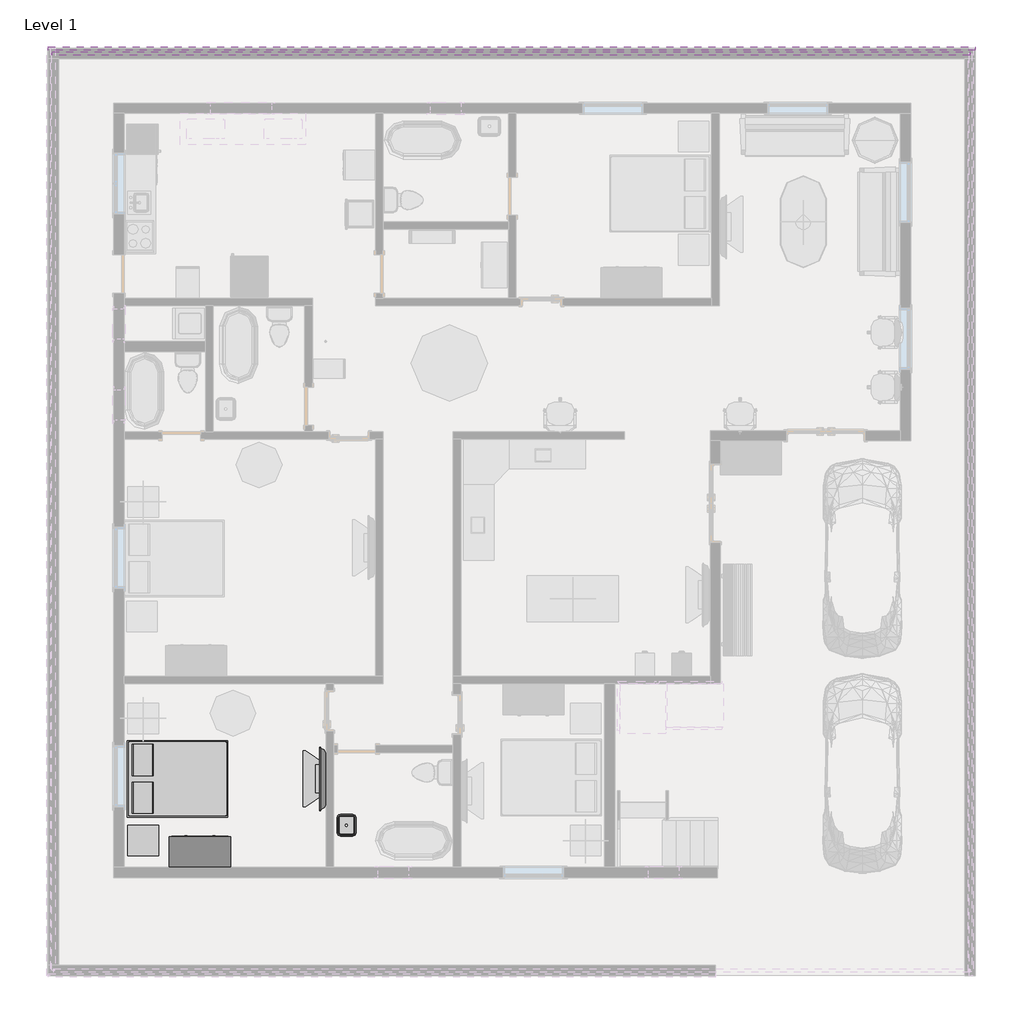
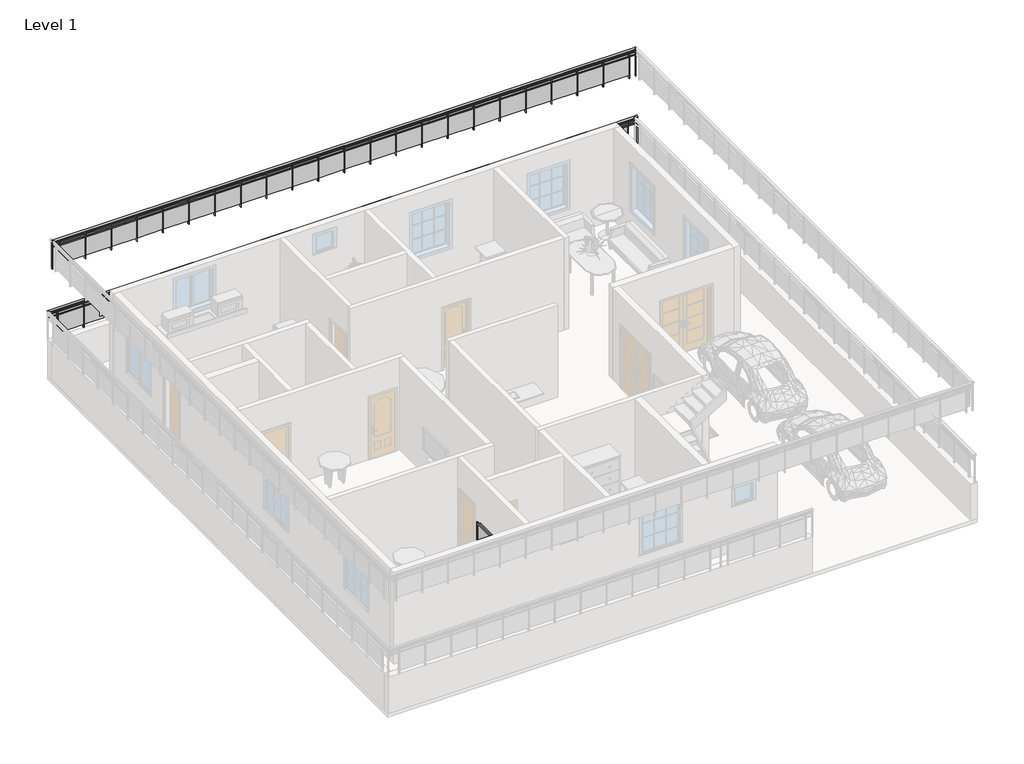
# One storey, part 5 of 6: 5 furniture elements, 2 railings, 1 flow terminal.
"""IFC4 building model written with IfcOpenShell, lengths in millimetres."""

from ifc_helpers import new_model, si_unit, point, frame, origin, place, context, project, spatial, polyline, ellipse_curve, trimmed, outline, extrude, transform, mapped, element, save
from ifc_brep_helpers import plane_surface, extruded_surface, advanced_brep
from components import flow_terminal_62a433f7, furniture_1d2926bd, furniture_9fa109b2, furniture_fdf74506, tv_stand_tv_stand_6ce107e5, furniture_5bc9ed15

model = new_model("IFC4")

# Units and contexts
model_context = context("Model", 3, world=origin())
ifc_project = project(units=[si_unit("LENGTHUNIT", "METRE", prefix="MILLI")], contexts=[model_context])

# Site, building, storey
site = spatial("IfcSite", under=ifc_project)
building = spatial("IfcBuilding", under=site)
storey = spatial("IfcBuildingStorey", under=building, Name="Level 1", Elevation=0.0)

# Flow terminal
placement = place(None, origin())
flow_terminal_shape = flow_terminal_62a433f7(model_context)
element("IfcFlowTerminal", 1, ObjectType="Sink Vanity-Square : 20\" x 18\"", at=placement, inside=storey, context=model_context, shape_type="MappedRepresentation", body=[
    mapped(flow_terminal_shape, transform((-1994.5948315, -1509.9134141, 609.6), x_axis=(0.0, 1.0000000000000004, 0.0), y_axis=(-1.0000000000000004, 0.0, 0.0), z_axis=(0.0, 0.0, 1.0))),
])

# Furniture
furniture_shape = furniture_1d2926bd(model_context)
element("IfcFurniture", 2, ObjectType="Bed-Box : Queen 60\" x 79\"", at=placement, inside=storey, context=model_context, shape_type="MappedRepresentation", body=[
    mapped(furniture_shape, transform((-5548.0082263, -906.2766325, 0.0), x_axis=(0.0, 1.0, 0.0), y_axis=(-1.0, 0.0, 0.0), z_axis=(0.0, 0.0, 1.0))),
])
furniture_2_shape = furniture_9fa109b2(model_context)
element("IfcFurniture", 3, ObjectType="Dresser : 48\" x 72\" x 24\"", at=placement, inside=storey, context=model_context, shape_type="MappedRepresentation", body=[
    mapped(furniture_2_shape, transform((-5136.3334924, -2390.7871276, 0.0), x_axis=(-1.0000000000000004, 0.0, 0.0), y_axis=(0.0, -1.0000000000000004, 0.0), z_axis=(0.0, 0.0, 1.0))),
])
furniture_3_shape = furniture_fdf74506(model_context)
element("IfcFurniture", 4, ObjectType="TV - Flat Screen : 50\"", at=placement, inside=storey, context=model_context, shape_type="MappedRepresentation", body=[
    mapped(furniture_3_shape, transform((-2411.0788562, -571.0686876, 914.4), x_axis=(0.0, -1.0, 0.0), y_axis=(1.0, 0.0, 0.0), z_axis=(0.0, 0.0, 1.0))),
])
tv_stand_tv_stand_shape = tv_stand_tv_stand_6ce107e5(model_context)
element("IfcFurniture", 5, ObjectType="TV Stand : TV Stand", at=placement, inside=storey, context=model_context, shape_type="MappedRepresentation", body=[
    mapped(tv_stand_tv_stand_shape, transform((-2352.5402326, -441.9361714, 0.0), x_axis=(0.0, -1.0, 0.0), y_axis=(1.0, 0.0, 0.0), z_axis=(0.0, 0.0, 1.0))),
])
furniture_4_shape = furniture_5bc9ed15(model_context)
element("IfcFurniture", 6, ObjectType="Table-Night Stand : 24\" x 24\" x 30\"", at=placement, inside=storey, context=model_context, shape_type="MappedRepresentation", body=[
    mapped(furniture_4_shape, transform((-6307.9123484, -2103.8241735, 0.0), x_axis=(1.0, 0.0, 0.0), y_axis=(0.0, 1.0, 0.0), z_axis=(0.0, 0.0, 1.0))),
])

# Railings
element("IfcRailing", 7, ObjectType="Glass Panel - Bottom Fill", at=placement, inside=storey, context=model_context, shape_type="SolidModel", body=[
    advanced_brep(
    [(10601.4597674, 13962.7633056, 2133.6), (10601.4597674, 14038.9633056, 2133.6), (-7889.7402326, 13962.7633056, 2133.6), (-7889.7402326, 14038.9633056, 2133.6)],
    [
        (0, 1, ellipse_curve(frame((10601.4597674, 14000.8633056, 2133.6), z_axis=(1.0, 0.0, 0.0), x_axis=(0.0, 1.0, 0.0)), 38.1, 28.575)),
        (1, 0, ellipse_curve(frame((10601.4597674, 14000.8633056, 2133.6), z_axis=(1.0, 0.0, 0.0), x_axis=(0.0, 1.0, 0.0)), 38.1, 28.575)),
        (2, 3, ellipse_curve(frame((-7889.7402326, 14000.8633056, 2133.6), z_axis=(-1.0, 0.0, 0.0), x_axis=(0.0, 1.0, 0.0)), 38.1, 28.575)),
        (3, 2, ellipse_curve(frame((-7889.7402326, 14000.8633056, 2133.6), z_axis=(-1.0, 0.0, 0.0), x_axis=(0.0, 1.0, 0.0)), 38.1, 28.575)),
        (0, 2),
        (3, 1),
    ],
    [
        plane_surface(frame((10601.4597674, 14000.8633056, 2133.6), z_axis=(1.0, 0.0, 0.0), x_axis=(0.0, -1.0, 0.0))),
        plane_surface(frame((-7889.7402326, 14000.8633056, 2133.6), z_axis=(-1.0, 0.0, 0.0), x_axis=(0.0, -1.0, 0.0))),
        extruded_surface(trimmed(ellipse_curve(frame((-7889.7402326, 14000.8633056, 2133.6), z_axis=(1.0, 0.0, 0.0), x_axis=(0.0, 1.0, 0.0)), 38.1, 28.575), [point((-7889.7402326, 13962.7633056, 2133.6))], [point((-7889.7402326, 14038.9633056, 2133.6))], True, "CARTESIAN"), (18491.2, 0.0, 0.0), 18491.2),
        extruded_surface(trimmed(ellipse_curve(frame((-7889.7402326, 14000.8633056, 2133.6), z_axis=(1.0, 0.0, 0.0), x_axis=(0.0, 1.0, 0.0)), 38.1, 28.575), [point((-7889.7402326, 14038.9633056, 2133.6))], [point((-7889.7402326, 13962.7633056, 2133.6))], True, "CARTESIAN"), (18491.2, 0.0, 0.0), 18491.2),
    ],
    [
        (0, [[1, 2]]),
        (1, [[3, 4]]),
        (2, [[-1, 5, -4, 6]]),
        (3, [[-2, -6, -3, -5]]),
    ],
),
    extrude(outline(polyline([(10601.4597674, 14013.5633056), (10601.4597674, 13988.1633056), (-7889.7402326, 13988.1633056), (-7889.7402326, 14013.5633056), (10601.4597674, 14013.5633056)])), frame((0.0, 0.0, 2019.3), z_axis=(0.0, 0.0, 1.0), x_axis=(1.0, 0.0, 0.0)), (0.0, 0.0, 1.0), 25.4),
    extrude(outline(polyline([(10601.4597674, 14013.5633056), (10601.4597674, 13988.1633056), (-7889.7402326, 13988.1633056), (-7889.7402326, 14013.5633056), (10601.4597674, 14013.5633056)])), frame((0.0, 0.0, 1917.7), z_axis=(0.0, 0.0, 1.0), x_axis=(1.0, 0.0, 0.0)), (0.0, 0.0, 1.0), 25.4),
    extrude(outline(polyline([(-7578.5902326, 14026.2633056), (-7578.5902326, 13975.4633056), (-7591.2902326, 13975.4633056), (-7591.2902326, 14026.2633056), (-7578.5902326, 14026.2633056)])), frame((0.0, 0.0, 1219.2), z_axis=(0.0, 0.0, 1.0), x_axis=(1.0, 0.0, 0.0)), (0.0, 0.0, 1.0), 885.6788223),
    extrude(outline(polyline([(-6772.1402326, 13994.3281486), (-7584.9402326, 13994.3281486), (-7584.9402326, 14000.6781486), (-6772.1402326, 14000.6781486), (-6772.1402326, 13994.3281486)])), frame((0.0, 0.0, 1320.8), z_axis=(0.0, 0.0, 1.0), x_axis=(1.0, 0.0, 0.0)), (0.0, 0.0, 1.0), 596.9),
    extrude(outline(polyline([(-6765.7902326, 14026.2633056), (-6765.7902326, 13975.4633056), (-6778.4902326, 13975.4633056), (-6778.4902326, 14026.2633056), (-6765.7902326, 14026.2633056)])), frame((0.0, 0.0, 1219.2), z_axis=(0.0, 0.0, 1.0), x_axis=(1.0, 0.0, 0.0)), (0.0, 0.0, 1.0), 885.6788223),
    extrude(outline(polyline([(-5959.3402326, 13994.3281486), (-6772.1402326, 13994.3281486), (-6772.1402326, 14000.6781486), (-5959.3402326, 14000.6781486), (-5959.3402326, 13994.3281486)])), frame((0.0, 0.0, 1320.8), z_axis=(0.0, 0.0, 1.0), x_axis=(1.0, 0.0, 0.0)), (0.0, 0.0, 1.0), 596.9),
    extrude(outline(polyline([(-5952.9902326, 14026.2633056), (-5952.9902326, 13975.4633056), (-5965.6902326, 13975.4633056), (-5965.6902326, 14026.2633056), (-5952.9902326, 14026.2633056)])), frame((0.0, 0.0, 1219.2), z_axis=(0.0, 0.0, 1.0), x_axis=(1.0, 0.0, 0.0)), (0.0, 0.0, 1.0), 885.6788223),
    extrude(outline(polyline([(-5146.5402326, 13994.3281486), (-5959.3402326, 13994.3281486), (-5959.3402326, 14000.6781486), (-5146.5402326, 14000.6781486), (-5146.5402326, 13994.3281486)])), frame((0.0, 0.0, 1320.8), z_axis=(0.0, 0.0, 1.0), x_axis=(1.0, 0.0, 0.0)), (0.0, 0.0, 1.0), 596.9),
    extrude(outline(polyline([(-5140.1902326, 14026.2633056), (-5140.1902326, 13975.4633056), (-5152.8902326, 13975.4633056), (-5152.8902326, 14026.2633056), (-5140.1902326, 14026.2633056)])), frame((0.0, 0.0, 1219.2), z_axis=(0.0, 0.0, 1.0), x_axis=(1.0, 0.0, 0.0)), (0.0, 0.0, 1.0), 885.6788223),
    extrude(outline(polyline([(-4333.7402326, 13994.3281486), (-5146.5402326, 13994.3281486), (-5146.5402326, 14000.6781486), (-4333.7402326, 14000.6781486), (-4333.7402326, 13994.3281486)])), frame((0.0, 0.0, 1320.8), z_axis=(0.0, 0.0, 1.0), x_axis=(1.0, 0.0, 0.0)), (0.0, 0.0, 1.0), 596.9),
    extrude(outline(polyline([(-4327.3902326, 14026.2633056), (-4327.3902326, 13975.4633056), (-4340.0902326, 13975.4633056), (-4340.0902326, 14026.2633056), (-4327.3902326, 14026.2633056)])), frame((0.0, 0.0, 1219.2), z_axis=(0.0, 0.0, 1.0), x_axis=(1.0, 0.0, 0.0)), (0.0, 0.0, 1.0), 885.6788223),
    extrude(outline(polyline([(-3520.9402326, 13994.3281486), (-4333.7402326, 13994.3281486), (-4333.7402326, 14000.6781486), (-3520.9402326, 14000.6781486), (-3520.9402326, 13994.3281486)])), frame((0.0, 0.0, 1320.8), z_axis=(0.0, 0.0, 1.0), x_axis=(1.0, 0.0, 0.0)), (0.0, 0.0, 1.0), 596.9),
    extrude(outline(polyline([(-3514.5902326, 14026.2633056), (-3514.5902326, 13975.4633056), (-3527.2902326, 13975.4633056), (-3527.2902326, 14026.2633056), (-3514.5902326, 14026.2633056)])), frame((0.0, 0.0, 1219.2), z_axis=(0.0, 0.0, 1.0), x_axis=(1.0, 0.0, 0.0)), (0.0, 0.0, 1.0), 885.6788223),
    extrude(outline(polyline([(-2708.1402326, 13994.3281486), (-3520.9402326, 13994.3281486), (-3520.9402326, 14000.6781486), (-2708.1402326, 14000.6781486), (-2708.1402326, 13994.3281486)])), frame((0.0, 0.0, 1320.8), z_axis=(0.0, 0.0, 1.0), x_axis=(1.0, 0.0, 0.0)), (0.0, 0.0, 1.0), 596.9),
    extrude(outline(polyline([(-2701.7902326, 14026.2633056), (-2701.7902326, 13975.4633056), (-2714.4902326, 13975.4633056), (-2714.4902326, 14026.2633056), (-2701.7902326, 14026.2633056)])), frame((0.0, 0.0, 1219.2), z_axis=(0.0, 0.0, 1.0), x_axis=(1.0, 0.0, 0.0)), (0.0, 0.0, 1.0), 885.6788223),
    extrude(outline(polyline([(-1895.3402326, 13994.3281486), (-2708.1402326, 13994.3281486), (-2708.1402326, 14000.6781486), (-1895.3402326, 14000.6781486), (-1895.3402326, 13994.3281486)])), frame((0.0, 0.0, 1320.8), z_axis=(0.0, 0.0, 1.0), x_axis=(1.0, 0.0, 0.0)), (0.0, 0.0, 1.0), 596.9),
    extrude(outline(polyline([(-1888.9902326, 14026.2633056), (-1888.9902326, 13975.4633056), (-1901.6902326, 13975.4633056), (-1901.6902326, 14026.2633056), (-1888.9902326, 14026.2633056)])), frame((0.0, 0.0, 1219.2), z_axis=(0.0, 0.0, 1.0), x_axis=(1.0, 0.0, 0.0)), (0.0, 0.0, 1.0), 885.6788223),
    extrude(outline(polyline([(-1082.5402326, 13994.3281486), (-1895.3402326, 13994.3281486), (-1895.3402326, 14000.6781486), (-1082.5402326, 14000.6781486), (-1082.5402326, 13994.3281486)])), frame((0.0, 0.0, 1320.8), z_axis=(0.0, 0.0, 1.0), x_axis=(1.0, 0.0, 0.0)), (0.0, 0.0, 1.0), 596.9),
    extrude(outline(polyline([(-1076.1902326, 14026.2633056), (-1076.1902326, 13975.4633056), (-1088.8902326, 13975.4633056), (-1088.8902326, 14026.2633056), (-1076.1902326, 14026.2633056)])), frame((0.0, 0.0, 1219.2), z_axis=(0.0, 0.0, 1.0), x_axis=(1.0, 0.0, 0.0)), (0.0, 0.0, 1.0), 885.6788223),
    extrude(outline(polyline([(-269.7402326, 13994.3281486), (-1082.5402326, 13994.3281486), (-1082.5402326, 14000.6781486), (-269.7402326, 14000.6781486), (-269.7402326, 13994.3281486)])), frame((0.0, 0.0, 1320.8), z_axis=(0.0, 0.0, 1.0), x_axis=(1.0, 0.0, 0.0)), (0.0, 0.0, 1.0), 596.9),
    extrude(outline(polyline([(-263.3902326, 14026.2633056), (-263.3902326, 13975.4633056), (-276.0902326, 13975.4633056), (-276.0902326, 14026.2633056), (-263.3902326, 14026.2633056)])), frame((0.0, 0.0, 1219.2), z_axis=(0.0, 0.0, 1.0), x_axis=(1.0, 0.0, 0.0)), (0.0, 0.0, 1.0), 885.6788223),
    extrude(outline(polyline([(543.0597674, 13994.3281486), (-269.7402326, 13994.3281486), (-269.7402326, 14000.6781486), (543.0597674, 14000.6781486), (543.0597674, 13994.3281486)])), frame((0.0, 0.0, 1320.8), z_axis=(0.0, 0.0, 1.0), x_axis=(1.0, 0.0, 0.0)), (0.0, 0.0, 1.0), 596.9),
    extrude(outline(polyline([(549.4097674, 14026.2633056), (549.4097674, 13975.4633056), (536.7097674, 13975.4633056), (536.7097674, 14026.2633056), (549.4097674, 14026.2633056)])), frame((0.0, 0.0, 1219.2), z_axis=(0.0, 0.0, 1.0), x_axis=(1.0, 0.0, 0.0)), (0.0, 0.0, 1.0), 885.6788223),
    extrude(outline(polyline([(1355.8597674, 13994.3281486), (543.0597674, 13994.3281486), (543.0597674, 14000.6781486), (1355.8597674, 14000.6781486), (1355.8597674, 13994.3281486)])), frame((0.0, 0.0, 1320.8), z_axis=(0.0, 0.0, 1.0), x_axis=(1.0, 0.0, 0.0)), (0.0, 0.0, 1.0), 596.9),
    extrude(outline(polyline([(1362.2097674, 14026.2633056), (1362.2097674, 13975.4633056), (1349.5097674, 13975.4633056), (1349.5097674, 14026.2633056), (1362.2097674, 14026.2633056)])), frame((0.0, 0.0, 1219.2), z_axis=(0.0, 0.0, 1.0), x_axis=(1.0, 0.0, 0.0)), (0.0, 0.0, 1.0), 885.6788223),
    extrude(outline(polyline([(2168.6597674, 13994.3281486), (1355.8597674, 13994.3281486), (1355.8597674, 14000.6781486), (2168.6597674, 14000.6781486), (2168.6597674, 13994.3281486)])), frame((0.0, 0.0, 1320.8), z_axis=(0.0, 0.0, 1.0), x_axis=(1.0, 0.0, 0.0)), (0.0, 0.0, 1.0), 596.9),
    extrude(outline(polyline([(2175.0097674, 14026.2633056), (2175.0097674, 13975.4633056), (2162.3097674, 13975.4633056), (2162.3097674, 14026.2633056), (2175.0097674, 14026.2633056)])), frame((0.0, 0.0, 1219.2), z_axis=(0.0, 0.0, 1.0), x_axis=(1.0, 0.0, 0.0)), (0.0, 0.0, 1.0), 885.6788223),
    extrude(outline(polyline([(2981.4597674, 13994.3281486), (2168.6597674, 13994.3281486), (2168.6597674, 14000.6781486), (2981.4597674, 14000.6781486), (2981.4597674, 13994.3281486)])), frame((0.0, 0.0, 1320.8), z_axis=(0.0, 0.0, 1.0), x_axis=(1.0, 0.0, 0.0)), (0.0, 0.0, 1.0), 596.9),
    extrude(outline(polyline([(2987.8097674, 14026.2633056), (2987.8097674, 13975.4633056), (2975.1097674, 13975.4633056), (2975.1097674, 14026.2633056), (2987.8097674, 14026.2633056)])), frame((0.0, 0.0, 1219.2), z_axis=(0.0, 0.0, 1.0), x_axis=(1.0, 0.0, 0.0)), (0.0, 0.0, 1.0), 885.6788223),
    extrude(outline(polyline([(3794.2597674, 13994.3281486), (2981.4597674, 13994.3281486), (2981.4597674, 14000.6781486), (3794.2597674, 14000.6781486), (3794.2597674, 13994.3281486)])), frame((0.0, 0.0, 1320.8), z_axis=(0.0, 0.0, 1.0), x_axis=(1.0, 0.0, 0.0)), (0.0, 0.0, 1.0), 596.9),
    extrude(outline(polyline([(3800.6097674, 14026.2633056), (3800.6097674, 13975.4633056), (3787.9097674, 13975.4633056), (3787.9097674, 14026.2633056), (3800.6097674, 14026.2633056)])), frame((0.0, 0.0, 1219.2), z_axis=(0.0, 0.0, 1.0), x_axis=(1.0, 0.0, 0.0)), (0.0, 0.0, 1.0), 885.6788223),
    extrude(outline(polyline([(4607.0597674, 13994.3281486), (3794.2597674, 13994.3281486), (3794.2597674, 14000.6781486), (4607.0597674, 14000.6781486), (4607.0597674, 13994.3281486)])), frame((0.0, 0.0, 1320.8), z_axis=(0.0, 0.0, 1.0), x_axis=(1.0, 0.0, 0.0)), (0.0, 0.0, 1.0), 596.9),
    extrude(outline(polyline([(4613.4097674, 14026.2633056), (4613.4097674, 13975.4633056), (4600.7097674, 13975.4633056), (4600.7097674, 14026.2633056), (4613.4097674, 14026.2633056)])), frame((0.0, 0.0, 1219.2), z_axis=(0.0, 0.0, 1.0), x_axis=(1.0, 0.0, 0.0)), (0.0, 0.0, 1.0), 885.6788223),
    extrude(outline(polyline([(5419.8597674, 13994.3281486), (4607.0597674, 13994.3281486), (4607.0597674, 14000.6781486), (5419.8597674, 14000.6781486), (5419.8597674, 13994.3281486)])), frame((0.0, 0.0, 1320.8), z_axis=(0.0, 0.0, 1.0), x_axis=(1.0, 0.0, 0.0)), (0.0, 0.0, 1.0), 596.9),
    extrude(outline(polyline([(5426.2097674, 14026.2633056), (5426.2097674, 13975.4633056), (5413.5097674, 13975.4633056), (5413.5097674, 14026.2633056), (5426.2097674, 14026.2633056)])), frame((0.0, 0.0, 1219.2), z_axis=(0.0, 0.0, 1.0), x_axis=(1.0, 0.0, 0.0)), (0.0, 0.0, 1.0), 885.6788223),
    extrude(outline(polyline([(6232.6597674, 13994.3281486), (5419.8597674, 13994.3281486), (5419.8597674, 14000.6781486), (6232.6597674, 14000.6781486), (6232.6597674, 13994.3281486)])), frame((0.0, 0.0, 1320.8), z_axis=(0.0, 0.0, 1.0), x_axis=(1.0, 0.0, 0.0)), (0.0, 0.0, 1.0), 596.9),
    extrude(outline(polyline([(6239.0097674, 14026.2633056), (6239.0097674, 13975.4633056), (6226.3097674, 13975.4633056), (6226.3097674, 14026.2633056), (6239.0097674, 14026.2633056)])), frame((0.0, 0.0, 1219.2), z_axis=(0.0, 0.0, 1.0), x_axis=(1.0, 0.0, 0.0)), (0.0, 0.0, 1.0), 885.6788223),
    extrude(outline(polyline([(7045.4597674, 13994.3281486), (6232.6597674, 13994.3281486), (6232.6597674, 14000.6781486), (7045.4597674, 14000.6781486), (7045.4597674, 13994.3281486)])), frame((0.0, 0.0, 1320.8), z_axis=(0.0, 0.0, 1.0), x_axis=(1.0, 0.0, 0.0)), (0.0, 0.0, 1.0), 596.9),
    extrude(outline(polyline([(7051.8097674, 14026.2633056), (7051.8097674, 13975.4633056), (7039.1097674, 13975.4633056), (7039.1097674, 14026.2633056), (7051.8097674, 14026.2633056)])), frame((0.0, 0.0, 1219.2), z_axis=(0.0, 0.0, 1.0), x_axis=(1.0, 0.0, 0.0)), (0.0, 0.0, 1.0), 885.6788223),
    extrude(outline(polyline([(7858.2597674, 13994.3281486), (7045.4597674, 13994.3281486), (7045.4597674, 14000.6781486), (7858.2597674, 14000.6781486), (7858.2597674, 13994.3281486)])), frame((0.0, 0.0, 1320.8), z_axis=(0.0, 0.0, 1.0), x_axis=(1.0, 0.0, 0.0)), (0.0, 0.0, 1.0), 596.9),
    extrude(outline(polyline([(7864.6097674, 14026.2633056), (7864.6097674, 13975.4633056), (7851.9097674, 13975.4633056), (7851.9097674, 14026.2633056), (7864.6097674, 14026.2633056)])), frame((0.0, 0.0, 1219.2), z_axis=(0.0, 0.0, 1.0), x_axis=(1.0, 0.0, 0.0)), (0.0, 0.0, 1.0), 885.6788223),
    extrude(outline(polyline([(8671.0597674, 13994.3281486), (7858.2597674, 13994.3281486), (7858.2597674, 14000.6781486), (8671.0597674, 14000.6781486), (8671.0597674, 13994.3281486)])), frame((0.0, 0.0, 1320.8), z_axis=(0.0, 0.0, 1.0), x_axis=(1.0, 0.0, 0.0)), (0.0, 0.0, 1.0), 596.9),
    extrude(outline(polyline([(8677.4097674, 14026.2633056), (8677.4097674, 13975.4633056), (8664.7097674, 13975.4633056), (8664.7097674, 14026.2633056), (8677.4097674, 14026.2633056)])), frame((0.0, 0.0, 1219.2), z_axis=(0.0, 0.0, 1.0), x_axis=(1.0, 0.0, 0.0)), (0.0, 0.0, 1.0), 885.6788223),
    extrude(outline(polyline([(9483.8597674, 13994.3281486), (8671.0597674, 13994.3281486), (8671.0597674, 14000.6781486), (9483.8597674, 14000.6781486), (9483.8597674, 13994.3281486)])), frame((0.0, 0.0, 1320.8), z_axis=(0.0, 0.0, 1.0), x_axis=(1.0, 0.0, 0.0)), (0.0, 0.0, 1.0), 596.9),
    extrude(outline(polyline([(9490.2097674, 14026.2633056), (9490.2097674, 13975.4633056), (9477.5097674, 13975.4633056), (9477.5097674, 14026.2633056), (9490.2097674, 14026.2633056)])), frame((0.0, 0.0, 1219.2), z_axis=(0.0, 0.0, 1.0), x_axis=(1.0, 0.0, 0.0)), (0.0, 0.0, 1.0), 885.6788223),
    extrude(outline(polyline([(10296.6597674, 13994.3281486), (9483.8597674, 13994.3281486), (9483.8597674, 14000.6781486), (10296.6597674, 14000.6781486), (10296.6597674, 13994.3281486)])), frame((0.0, 0.0, 1320.8), z_axis=(0.0, 0.0, 1.0), x_axis=(1.0, 0.0, 0.0)), (0.0, 0.0, 1.0), 596.9),
    extrude(outline(polyline([(10303.0097674, 14026.2633056), (10303.0097674, 13975.4633056), (10290.3097674, 13975.4633056), (10290.3097674, 14026.2633056), (10303.0097674, 14026.2633056)])), frame((0.0, 0.0, 1219.2), z_axis=(0.0, 0.0, 1.0), x_axis=(1.0, 0.0, 0.0)), (0.0, 0.0, 1.0), 885.6788223),
    extrude(outline(polyline([(-7877.0402326, 14010.3883056), (-7877.0402326, 13991.3383056), (-7896.0902326, 13991.3383056), (-7896.0902326, 14010.3883056), (-7877.0402326, 14010.3883056)])), frame((0.0, 0.0, 1219.2), z_axis=(0.0, 0.0, 1.0), x_axis=(1.0, 0.0, 0.0)), (0.0, 0.0, 1.0), 885.6788223),
    extrude(outline(polyline([(10607.8097674, 14010.3883056), (10607.8097674, 13991.3383056), (10588.7597674, 13991.3383056), (10588.7597674, 14010.3883056), (10607.8097674, 14010.3883056)])), frame((0.0, 0.0, 1219.2), z_axis=(0.0, 0.0, 1.0), x_axis=(1.0, 0.0, 0.0)), (0.0, 0.0, 1.0), 885.6788223),
])
element("IfcRailing", 8, ObjectType="Glass Panel - Bottom Fill", at=placement, inside=storey, context=model_context, shape_type="SolidModel", body=[
    advanced_brep(
    [(10499.8597674, 13861.1633056, 4495.8), (10499.8597674, 13937.3633056, 4495.8), (-7813.5402326, 13861.1633056, 4495.8), (-7813.5402326, 13937.3633056, 4495.8)],
    [
        (0, 1, ellipse_curve(frame((10499.8597674, 13899.2633056, 4495.8), z_axis=(1.0, 0.0, 0.0), x_axis=(0.0, 1.0, 0.0)), 38.1, 28.575)),
        (1, 0, ellipse_curve(frame((10499.8597674, 13899.2633056, 4495.8), z_axis=(1.0, 0.0, 0.0), x_axis=(0.0, 1.0, 0.0)), 38.1, 28.575)),
        (2, 3, ellipse_curve(frame((-7813.5402326, 13899.2633056, 4495.8), z_axis=(-1.0, 0.0, 0.0), x_axis=(0.0, 1.0, 0.0)), 38.1, 28.575)),
        (3, 2, ellipse_curve(frame((-7813.5402326, 13899.2633056, 4495.8), z_axis=(-1.0, 0.0, 0.0), x_axis=(0.0, 1.0, 0.0)), 38.1, 28.575)),
        (0, 2),
        (3, 1),
    ],
    [
        plane_surface(frame((10499.8597674, 13899.2633056, 4495.8), z_axis=(1.0, 0.0, 0.0), x_axis=(0.0, -1.0, 0.0))),
        plane_surface(frame((-7813.5402326, 13899.2633056, 4495.8), z_axis=(-1.0, 0.0, 0.0), x_axis=(0.0, -1.0, 0.0))),
        extruded_surface(trimmed(ellipse_curve(frame((-7813.5402326, 13899.2633056, 4495.8), z_axis=(1.0, 0.0, 0.0), x_axis=(0.0, 1.0, 0.0)), 38.1, 28.575), [point((-7813.5402326, 13861.1633056, 4495.8))], [point((-7813.5402326, 13937.3633056, 4495.8))], True, "CARTESIAN"), (18313.4, 0.0, 0.0), 18313.4),
        extruded_surface(trimmed(ellipse_curve(frame((-7813.5402326, 13899.2633056, 4495.8), z_axis=(1.0, 0.0, 0.0), x_axis=(0.0, 1.0, 0.0)), 38.1, 28.575), [point((-7813.5402326, 13937.3633056, 4495.8))], [point((-7813.5402326, 13861.1633056, 4495.8))], True, "CARTESIAN"), (18313.4, 0.0, 0.0), 18313.4),
    ],
    [
        (0, [[1, 2]]),
        (1, [[3, 4]]),
        (2, [[-1, 5, -4, 6]]),
        (3, [[-2, -6, -3, -5]]),
    ],
),
    extrude(outline(polyline([(10499.8597674, 13911.9633056), (10499.8597674, 13886.5633056), (-7813.5402326, 13886.5633056), (-7813.5402326, 13911.9633056), (10499.8597674, 13911.9633056)])), frame((0.0, 0.0, 4381.5), z_axis=(0.0, 0.0, 1.0), x_axis=(1.0, 0.0, 0.0)), (0.0, 0.0, 1.0), 25.4),
    extrude(outline(polyline([(10499.8597674, 13911.9633056), (10499.8597674, 13886.5633056), (-7813.5402326, 13886.5633056), (-7813.5402326, 13911.9633056), (10499.8597674, 13911.9633056)])), frame((0.0, 0.0, 4279.9), z_axis=(0.0, 0.0, 1.0), x_axis=(1.0, 0.0, 0.0)), (0.0, 0.0, 1.0), 25.4),
    extrude(outline(polyline([(-7591.2902326, 13924.6633056), (-7591.2902326, 13873.8633056), (-7603.9902326, 13873.8633056), (-7603.9902326, 13924.6633056), (-7591.2902326, 13924.6633056)])), frame((0.0, 0.0, 3581.4), z_axis=(0.0, 0.0, 1.0), x_axis=(1.0, 0.0, 0.0)), (0.0, 0.0, 1.0), 885.6788223),
    extrude(outline(polyline([(-6784.8402326, 13892.7281486), (-7597.6402326, 13892.7281486), (-7597.6402326, 13899.0781486), (-6784.8402326, 13899.0781486), (-6784.8402326, 13892.7281486)])), frame((0.0, 0.0, 3683.0), z_axis=(0.0, 0.0, 1.0), x_axis=(1.0, 0.0, 0.0)), (0.0, 0.0, 1.0), 596.9),
    extrude(outline(polyline([(-6778.4902326, 13924.6633056), (-6778.4902326, 13873.8633056), (-6791.1902326, 13873.8633056), (-6791.1902326, 13924.6633056), (-6778.4902326, 13924.6633056)])), frame((0.0, 0.0, 3581.4), z_axis=(0.0, 0.0, 1.0), x_axis=(1.0, 0.0, 0.0)), (0.0, 0.0, 1.0), 885.6788223),
    extrude(outline(polyline([(-5972.0402326, 13892.7281486), (-6784.8402326, 13892.7281486), (-6784.8402326, 13899.0781486), (-5972.0402326, 13899.0781486), (-5972.0402326, 13892.7281486)])), frame((0.0, 0.0, 3683.0), z_axis=(0.0, 0.0, 1.0), x_axis=(1.0, 0.0, 0.0)), (0.0, 0.0, 1.0), 596.9),
    extrude(outline(polyline([(-5965.6902326, 13924.6633056), (-5965.6902326, 13873.8633056), (-5978.3902326, 13873.8633056), (-5978.3902326, 13924.6633056), (-5965.6902326, 13924.6633056)])), frame((0.0, 0.0, 3581.4), z_axis=(0.0, 0.0, 1.0), x_axis=(1.0, 0.0, 0.0)), (0.0, 0.0, 1.0), 885.6788223),
    extrude(outline(polyline([(-5159.2402326, 13892.7281486), (-5972.0402326, 13892.7281486), (-5972.0402326, 13899.0781486), (-5159.2402326, 13899.0781486), (-5159.2402326, 13892.7281486)])), frame((0.0, 0.0, 3683.0), z_axis=(0.0, 0.0, 1.0), x_axis=(1.0, 0.0, 0.0)), (0.0, 0.0, 1.0), 596.9),
    extrude(outline(polyline([(-5152.8902326, 13924.6633056), (-5152.8902326, 13873.8633056), (-5165.5902326, 13873.8633056), (-5165.5902326, 13924.6633056), (-5152.8902326, 13924.6633056)])), frame((0.0, 0.0, 3581.4), z_axis=(0.0, 0.0, 1.0), x_axis=(1.0, 0.0, 0.0)), (0.0, 0.0, 1.0), 885.6788223),
    extrude(outline(polyline([(-4346.4402326, 13892.7281486), (-5159.2402326, 13892.7281486), (-5159.2402326, 13899.0781486), (-4346.4402326, 13899.0781486), (-4346.4402326, 13892.7281486)])), frame((0.0, 0.0, 3683.0), z_axis=(0.0, 0.0, 1.0), x_axis=(1.0, 0.0, 0.0)), (0.0, 0.0, 1.0), 596.9),
    extrude(outline(polyline([(-4340.0902326, 13924.6633056), (-4340.0902326, 13873.8633056), (-4352.7902326, 13873.8633056), (-4352.7902326, 13924.6633056), (-4340.0902326, 13924.6633056)])), frame((0.0, 0.0, 3581.4), z_axis=(0.0, 0.0, 1.0), x_axis=(1.0, 0.0, 0.0)), (0.0, 0.0, 1.0), 885.6788223),
    extrude(outline(polyline([(-3533.6402326, 13892.7281486), (-4346.4402326, 13892.7281486), (-4346.4402326, 13899.0781486), (-3533.6402326, 13899.0781486), (-3533.6402326, 13892.7281486)])), frame((0.0, 0.0, 3683.0), z_axis=(0.0, 0.0, 1.0), x_axis=(1.0, 0.0, 0.0)), (0.0, 0.0, 1.0), 596.9),
    extrude(outline(polyline([(-3527.2902326, 13924.6633056), (-3527.2902326, 13873.8633056), (-3539.9902326, 13873.8633056), (-3539.9902326, 13924.6633056), (-3527.2902326, 13924.6633056)])), frame((0.0, 0.0, 3581.4), z_axis=(0.0, 0.0, 1.0), x_axis=(1.0, 0.0, 0.0)), (0.0, 0.0, 1.0), 885.6788223),
    extrude(outline(polyline([(-2720.8402326, 13892.7281486), (-3533.6402326, 13892.7281486), (-3533.6402326, 13899.0781486), (-2720.8402326, 13899.0781486), (-2720.8402326, 13892.7281486)])), frame((0.0, 0.0, 3683.0), z_axis=(0.0, 0.0, 1.0), x_axis=(1.0, 0.0, 0.0)), (0.0, 0.0, 1.0), 596.9),
    extrude(outline(polyline([(-2714.4902326, 13924.6633056), (-2714.4902326, 13873.8633056), (-2727.1902326, 13873.8633056), (-2727.1902326, 13924.6633056), (-2714.4902326, 13924.6633056)])), frame((0.0, 0.0, 3581.4), z_axis=(0.0, 0.0, 1.0), x_axis=(1.0, 0.0, 0.0)), (0.0, 0.0, 1.0), 885.6788223),
    extrude(outline(polyline([(-1908.0402326, 13892.7281486), (-2720.8402326, 13892.7281486), (-2720.8402326, 13899.0781486), (-1908.0402326, 13899.0781486), (-1908.0402326, 13892.7281486)])), frame((0.0, 0.0, 3683.0), z_axis=(0.0, 0.0, 1.0), x_axis=(1.0, 0.0, 0.0)), (0.0, 0.0, 1.0), 596.9),
    extrude(outline(polyline([(-1901.6902326, 13924.6633056), (-1901.6902326, 13873.8633056), (-1914.3902326, 13873.8633056), (-1914.3902326, 13924.6633056), (-1901.6902326, 13924.6633056)])), frame((0.0, 0.0, 3581.4), z_axis=(0.0, 0.0, 1.0), x_axis=(1.0, 0.0, 0.0)), (0.0, 0.0, 1.0), 885.6788223),
    extrude(outline(polyline([(-1095.2402326, 13892.7281486), (-1908.0402326, 13892.7281486), (-1908.0402326, 13899.0781486), (-1095.2402326, 13899.0781486), (-1095.2402326, 13892.7281486)])), frame((0.0, 0.0, 3683.0), z_axis=(0.0, 0.0, 1.0), x_axis=(1.0, 0.0, 0.0)), (0.0, 0.0, 1.0), 596.9),
    extrude(outline(polyline([(-1088.8902326, 13924.6633056), (-1088.8902326, 13873.8633056), (-1101.5902326, 13873.8633056), (-1101.5902326, 13924.6633056), (-1088.8902326, 13924.6633056)])), frame((0.0, 0.0, 3581.4), z_axis=(0.0, 0.0, 1.0), x_axis=(1.0, 0.0, 0.0)), (0.0, 0.0, 1.0), 885.6788223),
    extrude(outline(polyline([(-282.4402326, 13892.7281486), (-1095.2402326, 13892.7281486), (-1095.2402326, 13899.0781486), (-282.4402326, 13899.0781486), (-282.4402326, 13892.7281486)])), frame((0.0, 0.0, 3683.0), z_axis=(0.0, 0.0, 1.0), x_axis=(1.0, 0.0, 0.0)), (0.0, 0.0, 1.0), 596.9),
    extrude(outline(polyline([(-276.0902326, 13924.6633056), (-276.0902326, 13873.8633056), (-288.7902326, 13873.8633056), (-288.7902326, 13924.6633056), (-276.0902326, 13924.6633056)])), frame((0.0, 0.0, 3581.4), z_axis=(0.0, 0.0, 1.0), x_axis=(1.0, 0.0, 0.0)), (0.0, 0.0, 1.0), 885.6788223),
    extrude(outline(polyline([(530.3597674, 13892.7281486), (-282.4402326, 13892.7281486), (-282.4402326, 13899.0781486), (530.3597674, 13899.0781486), (530.3597674, 13892.7281486)])), frame((0.0, 0.0, 3683.0), z_axis=(0.0, 0.0, 1.0), x_axis=(1.0, 0.0, 0.0)), (0.0, 0.0, 1.0), 596.9),
    extrude(outline(polyline([(536.7097674, 13924.6633056), (536.7097674, 13873.8633056), (524.0097674, 13873.8633056), (524.0097674, 13924.6633056), (536.7097674, 13924.6633056)])), frame((0.0, 0.0, 3581.4), z_axis=(0.0, 0.0, 1.0), x_axis=(1.0, 0.0, 0.0)), (0.0, 0.0, 1.0), 885.6788223),
    extrude(outline(polyline([(1343.1597674, 13892.7281486), (530.3597674, 13892.7281486), (530.3597674, 13899.0781486), (1343.1597674, 13899.0781486), (1343.1597674, 13892.7281486)])), frame((0.0, 0.0, 3683.0), z_axis=(0.0, 0.0, 1.0), x_axis=(1.0, 0.0, 0.0)), (0.0, 0.0, 1.0), 596.9),
    extrude(outline(polyline([(1349.5097674, 13924.6633056), (1349.5097674, 13873.8633056), (1336.8097674, 13873.8633056), (1336.8097674, 13924.6633056), (1349.5097674, 13924.6633056)])), frame((0.0, 0.0, 3581.4), z_axis=(0.0, 0.0, 1.0), x_axis=(1.0, 0.0, 0.0)), (0.0, 0.0, 1.0), 885.6788223),
    extrude(outline(polyline([(2155.9597674, 13892.7281486), (1343.1597674, 13892.7281486), (1343.1597674, 13899.0781486), (2155.9597674, 13899.0781486), (2155.9597674, 13892.7281486)])), frame((0.0, 0.0, 3683.0), z_axis=(0.0, 0.0, 1.0), x_axis=(1.0, 0.0, 0.0)), (0.0, 0.0, 1.0), 596.9),
    extrude(outline(polyline([(2162.3097674, 13924.6633056), (2162.3097674, 13873.8633056), (2149.6097674, 13873.8633056), (2149.6097674, 13924.6633056), (2162.3097674, 13924.6633056)])), frame((0.0, 0.0, 3581.4), z_axis=(0.0, 0.0, 1.0), x_axis=(1.0, 0.0, 0.0)), (0.0, 0.0, 1.0), 885.6788223),
    extrude(outline(polyline([(2968.7597674, 13892.7281486), (2155.9597674, 13892.7281486), (2155.9597674, 13899.0781486), (2968.7597674, 13899.0781486), (2968.7597674, 13892.7281486)])), frame((0.0, 0.0, 3683.0), z_axis=(0.0, 0.0, 1.0), x_axis=(1.0, 0.0, 0.0)), (0.0, 0.0, 1.0), 596.9),
    extrude(outline(polyline([(2975.1097674, 13924.6633056), (2975.1097674, 13873.8633056), (2962.4097674, 13873.8633056), (2962.4097674, 13924.6633056), (2975.1097674, 13924.6633056)])), frame((0.0, 0.0, 3581.4), z_axis=(0.0, 0.0, 1.0), x_axis=(1.0, 0.0, 0.0)), (0.0, 0.0, 1.0), 885.6788223),
    extrude(outline(polyline([(3781.5597674, 13892.7281486), (2968.7597674, 13892.7281486), (2968.7597674, 13899.0781486), (3781.5597674, 13899.0781486), (3781.5597674, 13892.7281486)])), frame((0.0, 0.0, 3683.0), z_axis=(0.0, 0.0, 1.0), x_axis=(1.0, 0.0, 0.0)), (0.0, 0.0, 1.0), 596.9),
    extrude(outline(polyline([(3787.9097674, 13924.6633056), (3787.9097674, 13873.8633056), (3775.2097674, 13873.8633056), (3775.2097674, 13924.6633056), (3787.9097674, 13924.6633056)])), frame((0.0, 0.0, 3581.4), z_axis=(0.0, 0.0, 1.0), x_axis=(1.0, 0.0, 0.0)), (0.0, 0.0, 1.0), 885.6788223),
    extrude(outline(polyline([(4594.3597674, 13892.7281486), (3781.5597674, 13892.7281486), (3781.5597674, 13899.0781486), (4594.3597674, 13899.0781486), (4594.3597674, 13892.7281486)])), frame((0.0, 0.0, 3683.0), z_axis=(0.0, 0.0, 1.0), x_axis=(1.0, 0.0, 0.0)), (0.0, 0.0, 1.0), 596.9),
    extrude(outline(polyline([(4600.7097674, 13924.6633056), (4600.7097674, 13873.8633056), (4588.0097674, 13873.8633056), (4588.0097674, 13924.6633056), (4600.7097674, 13924.6633056)])), frame((0.0, 0.0, 3581.4), z_axis=(0.0, 0.0, 1.0), x_axis=(1.0, 0.0, 0.0)), (0.0, 0.0, 1.0), 885.6788223),
    extrude(outline(polyline([(5407.1597674, 13892.7281486), (4594.3597674, 13892.7281486), (4594.3597674, 13899.0781486), (5407.1597674, 13899.0781486), (5407.1597674, 13892.7281486)])), frame((0.0, 0.0, 3683.0), z_axis=(0.0, 0.0, 1.0), x_axis=(1.0, 0.0, 0.0)), (0.0, 0.0, 1.0), 596.9),
    extrude(outline(polyline([(5413.5097674, 13924.6633056), (5413.5097674, 13873.8633056), (5400.8097674, 13873.8633056), (5400.8097674, 13924.6633056), (5413.5097674, 13924.6633056)])), frame((0.0, 0.0, 3581.4), z_axis=(0.0, 0.0, 1.0), x_axis=(1.0, 0.0, 0.0)), (0.0, 0.0, 1.0), 885.6788223),
    extrude(outline(polyline([(6219.9597674, 13892.7281486), (5407.1597674, 13892.7281486), (5407.1597674, 13899.0781486), (6219.9597674, 13899.0781486), (6219.9597674, 13892.7281486)])), frame((0.0, 0.0, 3683.0), z_axis=(0.0, 0.0, 1.0), x_axis=(1.0, 0.0, 0.0)), (0.0, 0.0, 1.0), 596.9),
    extrude(outline(polyline([(6226.3097674, 13924.6633056), (6226.3097674, 13873.8633056), (6213.6097674, 13873.8633056), (6213.6097674, 13924.6633056), (6226.3097674, 13924.6633056)])), frame((0.0, 0.0, 3581.4), z_axis=(0.0, 0.0, 1.0), x_axis=(1.0, 0.0, 0.0)), (0.0, 0.0, 1.0), 885.6788223),
    extrude(outline(polyline([(7032.7597674, 13892.7281486), (6219.9597674, 13892.7281486), (6219.9597674, 13899.0781486), (7032.7597674, 13899.0781486), (7032.7597674, 13892.7281486)])), frame((0.0, 0.0, 3683.0), z_axis=(0.0, 0.0, 1.0), x_axis=(1.0, 0.0, 0.0)), (0.0, 0.0, 1.0), 596.9),
    extrude(outline(polyline([(7039.1097674, 13924.6633056), (7039.1097674, 13873.8633056), (7026.4097674, 13873.8633056), (7026.4097674, 13924.6633056), (7039.1097674, 13924.6633056)])), frame((0.0, 0.0, 3581.4), z_axis=(0.0, 0.0, 1.0), x_axis=(1.0, 0.0, 0.0)), (0.0, 0.0, 1.0), 885.6788223),
    extrude(outline(polyline([(7845.5597674, 13892.7281486), (7032.7597674, 13892.7281486), (7032.7597674, 13899.0781486), (7845.5597674, 13899.0781486), (7845.5597674, 13892.7281486)])), frame((0.0, 0.0, 3683.0), z_axis=(0.0, 0.0, 1.0), x_axis=(1.0, 0.0, 0.0)), (0.0, 0.0, 1.0), 596.9),
    extrude(outline(polyline([(7851.9097674, 13924.6633056), (7851.9097674, 13873.8633056), (7839.2097674, 13873.8633056), (7839.2097674, 13924.6633056), (7851.9097674, 13924.6633056)])), frame((0.0, 0.0, 3581.4), z_axis=(0.0, 0.0, 1.0), x_axis=(1.0, 0.0, 0.0)), (0.0, 0.0, 1.0), 885.6788223),
    extrude(outline(polyline([(8658.3597674, 13892.7281486), (7845.5597674, 13892.7281486), (7845.5597674, 13899.0781486), (8658.3597674, 13899.0781486), (8658.3597674, 13892.7281486)])), frame((0.0, 0.0, 3683.0), z_axis=(0.0, 0.0, 1.0), x_axis=(1.0, 0.0, 0.0)), (0.0, 0.0, 1.0), 596.9),
    extrude(outline(polyline([(8664.7097674, 13924.6633056), (8664.7097674, 13873.8633056), (8652.0097674, 13873.8633056), (8652.0097674, 13924.6633056), (8664.7097674, 13924.6633056)])), frame((0.0, 0.0, 3581.4), z_axis=(0.0, 0.0, 1.0), x_axis=(1.0, 0.0, 0.0)), (0.0, 0.0, 1.0), 885.6788223),
    extrude(outline(polyline([(9471.1597674, 13892.7281486), (8658.3597674, 13892.7281486), (8658.3597674, 13899.0781486), (9471.1597674, 13899.0781486), (9471.1597674, 13892.7281486)])), frame((0.0, 0.0, 3683.0), z_axis=(0.0, 0.0, 1.0), x_axis=(1.0, 0.0, 0.0)), (0.0, 0.0, 1.0), 596.9),
    extrude(outline(polyline([(9477.5097674, 13924.6633056), (9477.5097674, 13873.8633056), (9464.8097674, 13873.8633056), (9464.8097674, 13924.6633056), (9477.5097674, 13924.6633056)])), frame((0.0, 0.0, 3581.4), z_axis=(0.0, 0.0, 1.0), x_axis=(1.0, 0.0, 0.0)), (0.0, 0.0, 1.0), 885.6788223),
    extrude(outline(polyline([(10283.9597674, 13892.7281486), (9471.1597674, 13892.7281486), (9471.1597674, 13899.0781486), (10283.9597674, 13899.0781486), (10283.9597674, 13892.7281486)])), frame((0.0, 0.0, 3683.0), z_axis=(0.0, 0.0, 1.0), x_axis=(1.0, 0.0, 0.0)), (0.0, 0.0, 1.0), 596.9),
    extrude(outline(polyline([(10290.3097674, 13924.6633056), (10290.3097674, 13873.8633056), (10277.6097674, 13873.8633056), (10277.6097674, 13924.6633056), (10290.3097674, 13924.6633056)])), frame((0.0, 0.0, 3581.4), z_axis=(0.0, 0.0, 1.0), x_axis=(1.0, 0.0, 0.0)), (0.0, 0.0, 1.0), 885.6788223),
    extrude(outline(polyline([(-7800.8402326, 13908.7883056), (-7800.8402326, 13889.7383056), (-7819.8902326, 13889.7383056), (-7819.8902326, 13908.7883056), (-7800.8402326, 13908.7883056)])), frame((0.0, 0.0, 3581.4), z_axis=(0.0, 0.0, 1.0), x_axis=(1.0, 0.0, 0.0)), (0.0, 0.0, 1.0), 885.6788223),
    extrude(outline(polyline([(10506.2097674, 13908.7883056), (10506.2097674, 13889.7383056), (10487.1597674, 13889.7383056), (10487.1597674, 13908.7883056), (10506.2097674, 13908.7883056)])), frame((0.0, 0.0, 3581.4), z_axis=(0.0, 0.0, 1.0), x_axis=(1.0, 0.0, 0.0)), (0.0, 0.0, 1.0), 885.6788223),
])

save(model, "model.ifc")

# Revit data of these elements
# Type "Sink Vanity-Square : 20\" x 18\""
#   Assembly Code = "D2010400"
#   Counter Height = 2' - 7"
#   Depth = 1' - 6"
#   Width = 1' - 8"
#   Basin Material = Porcelain, Linen
#   Faucet Material = Steel, Polished
#   Default Elevation = 0
# Type "Bed-Box : Queen 60\" x 79\""
#   Assembly Code = "E2020200"
#   Length = 6' - 7"
#   Width = 5' - 0"
#   Frame Material = Birch
#   Mattress Material = Linen, White
#   Default Elevation = 0
# Type "Dresser : 48\" x 72\" x 24\""
#   Assembly Code = "E2020200"
#   Depth = 2' - 0"
#   Height = 6' - 0"
#   Width = 4' - 0"
#   Dresser Material = Laminate - Ivory, Glossy
#   Drawer Material = Laminate, Ivory, Matte
#   Knob Material = Cherry
#   Default Elevation = 0
# Type "TV - Flat Screen : 50\""
#   SinAng = 0' - 0.0193"
#   L = 3' - 7.57782"
#   H = 2' - 0.51477"
#   Thickness = 0' - 4.33071"
#   Diagonal = 4' - 2"
#   CosAng = 0' - 0.03431"
#   Stand [instance default] = yes
#   Default Elevation = 0
# Type "TV Stand : TV Stand"
#   Depth = 1' - 6"
#   Width = 3' - 8"
#   Height = 1' - 7 1/2"
#   Finish = Melamine - Gray
#   Default Elevation = 0
# Type "Table-Night Stand : 24\" x 24\" x 30\""
#   Assembly Code = "E2020200"
#   Depth = 2' - 0"
#   Height = 2' - 6"
#   Width = 2' - 0"
#   Base Material = Birch
#   Top Material = Laminate, Ivory, Matte
#   Default Elevation = 0
# Type "Glass Panel - Bottom Fill"
#   Assembly Code = "C2010400"
#   built-in parameter 1008612 = 0.0416667 (stored number, unit not read)
#   built-in parameter 1008611 = 0.0416667 (stored number, unit not read)
#   built-in parameter 1008609 = 0.333333 (stored number, unit not read)
#   built-in parameter 1008604 = 0.166667 (stored number, unit not read)
#   built-in parameter 1008603 = 0.166667 (stored number, unit not read)
#   Railing Height = 3' - 0"
#   built-in parameter 1008630 = 2
#   built-in parameter 1008610 = 2
#   built-in parameter 1008618 = Baluster - Square : 3/4"
# Element 1 (IfcFlowTerminal, "Sink Vanity-Square : 20\" x 18\"")
#   Mark = "10"
#   Phase Created = New Construction
#   Materials on its faces: "Porcelain, Linen", "Steel, Polished"
# Element 2 (IfcFurniture, "Bed-Box : Queen 60\" x 79\"")
#   Phase Created = New Construction
#   Materials on its faces: "Birch", "Linen, White"
# Element 3 (IfcFurniture, "Dresser : 48\" x 72\" x 24\"")
#   Phase Created = New Construction
#   Materials on its faces: "Laminate, Ivory, Matte", "Cherry", "Laminate - Ivory, Glossy"
# Element 4 (IfcFurniture, "TV - Flat Screen : 50\"")
#   Stand = yes
#   Phase Created = New Construction
#   Materials on its faces: "TV - Black", "TV - Glass", "TV - Screen"
# Element 5 (IfcFurniture, "TV Stand : TV Stand")
#   Phase Created = New Construction
#   Materials on its faces: "Melamine - Gray", "Glass - Shelves"
# Element 6 (IfcFurniture, "Table-Night Stand : 24\" x 24\" x 30\"")
#   Phase Created = New Construction
#   Materials on its faces: "Birch", "Laminate, Ivory, Matte"
# Element 7 (IfcRailing, "Glass Panel - Bottom Fill")
#   built-in parameter 1008621 = 4 (stored number, unit not read)
#   Phase Created = New Construction
#   Materials on its faces: "Glass"
# Element 8 (IfcRailing, "Glass Panel - Bottom Fill")
#   built-in parameter 1008621 = 11.75 (stored number, unit not read)
#   Phase Created = New Construction
#   Materials on its faces: "Glass"
# Materials
#   "Porcelain, Linen": class "Ceramic", colour RGB 249 239 230, transparency 0, Description = "Porcelain, linen", Cost = 0
#   "Steel, Polished": class "Metal", colour RGB 57 57 57, transparency 0, Description = "Polished steel", Cost = 0
#   "Birch": class "Wood", colour RGB 224 178 126, transparency 0, Description = "Betula Alleghaniensis", Cost = 0
#   "Linen, White": class "Textile", colour RGB 247 247 239, transparency 0, Description = "Linen, white", Cost = 0
#   "Laminate - Ivory, Glossy": colour RGB 247 247 239, transparency 0
#   "Laminate, Ivory, Matte": class "Plastic", colour RGB 247 247 239, transparency 0, Description = "Plastic Laminate - Ivory, Matte", Cost = 0
#   "Cherry": class "Wood", colour RGB 226 177 128, transparency 0, Description = "Prunus Serotina", Cost = 0
#   "Melamine - Gray": class "Wood", colour RGB 49 49 49, transparency 0
#   "TV - Black": colour RGB 49 49 49, transparency 0
#   "TV - Glass": colour RGB 157 157 157, transparency 0.9
#   "TV - Screen": colour RGB 0 0 0, transparency 0
#   "Glass - Shelves": class "Glass", colour RGB 167 167 167, transparency 0.9
#   "Glass": class "Glass", colour RGB 0 128 192, transparency 0.75, Description = "Soda Lime Glass", Cost = 0
